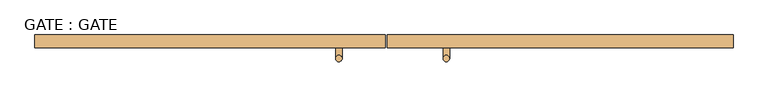
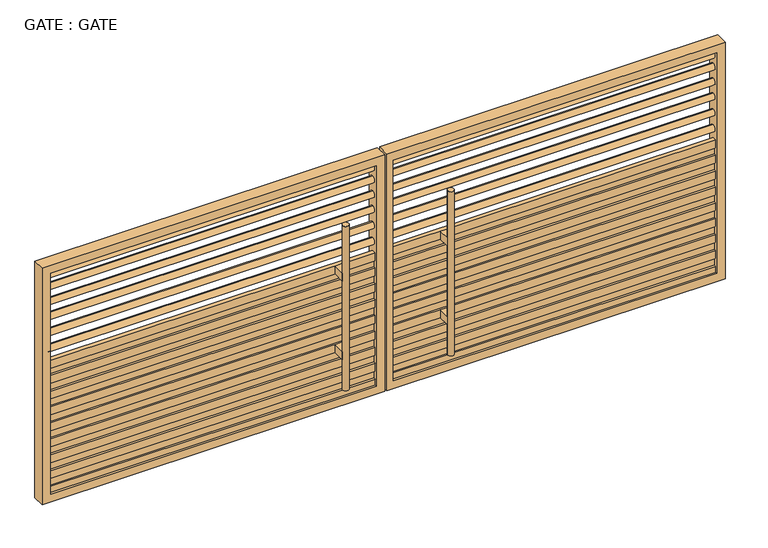
"""IFC4 building model written with IfcOpenShell, lengths in millimetres: door geometry, GATE : GATE."""

from ifc_helpers import new_model, si_unit, point, frame, frame_2d, origin, place, context, project, spatial, polyline, circle_curve, trimmed, segment, composite_curve, outline, extrude, source, transform, mapped, element, save


def gate_gate_6d9155c2(model_context):
    return source(origin(), model_context, "Body", "SweptSolid", [
        extrude(outline(composite_curve([segment(trimmed(circle_curve(frame_2d((-3297.4327882, -6020.0544725)), 19.05), [point((-3316.4827882, -6020.0544725))], [point((-3278.3827882, -6020.0544725))], False, "CARTESIAN"), True, "CONTINUOUS"), segment(trimmed(circle_curve(frame_2d((-3297.4327882, -6020.0544725)), 19.05), [point((-3278.3827882, -6020.0544725))], [point((-3316.4827882, -6020.0544725))], False, "CARTESIAN"), True, "CONTINUOUS")], self_intersect=False)), frame((0.0, 0.0, 202.6054074), z_axis=(0.0, 0.0, 1.0), x_axis=(1.0, 0.0, 0.0)), (0.0, 0.0, 1.0), 1048.3445926),
        extrude(outline(polyline([(-3278.3827882, -6020.0544725), (-3316.4827882, -6020.0544725), (-3316.4827882, -5943.8544725), (-3278.3827882, -5943.8544725), (-3278.3827882, -6020.0544725)])), frame((0.0, 0.0, 895.35), z_axis=(0.0, 0.0, 1.0), x_axis=(1.0, 0.0, 0.0)), (0.0, 0.0, 1.0), 50.8),
        extrude(outline(polyline([(-3278.3827882, -6020.0544725), (-3316.4827882, -6020.0544725), (-3316.4827882, -5943.8544725), (-3278.3827882, -5943.8544725), (-3278.3827882, -6020.0544725)])), frame((0.0, 0.0, 393.7), z_axis=(0.0, 0.0, 1.0), x_axis=(1.0, 0.0, 0.0)), (0.0, 0.0, 1.0), 50.8),
        extrude(outline(composite_curve([segment(trimmed(circle_curve(frame_2d((-3932.4327882, -6020.0544725)), 19.05), [point((-3951.4827882, -6020.0544725))], [point((-3913.3827882, -6020.0544725))], False, "CARTESIAN"), True, "CONTINUOUS"), segment(trimmed(circle_curve(frame_2d((-3932.4327882, -6020.0544725)), 19.05), [point((-3913.3827882, -6020.0544725))], [point((-3951.4827882, -6020.0544725))], False, "CARTESIAN"), True, "CONTINUOUS")], self_intersect=False)), frame((0.0, 0.0, 202.6054074), z_axis=(0.0, 0.0, 1.0), x_axis=(1.0, 0.0, 0.0)), (0.0, 0.0, 1.0), 1048.3445926),
        extrude(outline(polyline([(-3913.3827882, -6020.0544725), (-3951.4827882, -6020.0544725), (-3951.4827882, -5943.8544725), (-3913.3827882, -5943.8544725), (-3913.3827882, -6020.0544725)])), frame((0.0, 0.0, 895.35), z_axis=(0.0, 0.0, 1.0), x_axis=(1.0, 0.0, 0.0)), (0.0, 0.0, 1.0), 50.8),
        extrude(outline(polyline([(-3913.3827882, -6020.0544725), (-3951.4827882, -6020.0544725), (-3951.4827882, -5943.8544725), (-3913.3827882, -5943.8544725), (-3913.3827882, -6020.0544725)])), frame((0.0, 0.0, 393.7), z_axis=(0.0, 0.0, 1.0), x_axis=(1.0, 0.0, 0.0)), (0.0, 0.0, 1.0), 50.8),
        extrude(outline(polyline([(-5918.4544725, 946.15), (-5918.4544725, 101.6), (-5943.8544725, 101.6), (-5943.8544725, 139.7), (-5931.1544725, 139.7), (-5931.1544725, 190.5), (-5943.8544725, 190.5), (-5943.8544725, 241.3), (-5931.1544725, 241.3), (-5931.1544725, 292.1), (-5943.8544725, 292.1), (-5943.8544725, 342.9), (-5931.1544725, 342.9), (-5931.1544725, 393.7), (-5943.8544725, 393.7), (-5943.8544725, 444.5), (-5931.1544725, 444.5), (-5931.1544725, 495.3), (-5943.8544725, 495.3), (-5943.8544725, 546.1), (-5931.1544725, 546.1), (-5931.1544725, 596.9), (-5943.8544725, 596.9), (-5943.8544725, 647.7), (-5931.1544725, 647.7), (-5931.1544725, 698.5), (-5943.8544725, 698.5), (-5943.8544725, 749.3), (-5931.1544725, 749.3), (-5931.1544725, 800.1), (-5943.8544725, 800.1), (-5943.8544725, 850.9), (-5931.1544725, 850.9), (-5931.1544725, 895.35), (-5943.8544725, 895.35), (-5943.8544725, 946.15), (-5918.4544725, 946.15)])), frame((-3608.5827882, 0.0, 0.0), z_axis=(1.0, 0.0, 0.0), x_axis=(0.0, 1.0, 0.0)), (0.0, 0.0, 1.0), 1968.1845842),
        extrude(outline(composite_curve([segment(trimmed(circle_curve(frame_2d((-5918.4544725, 1479.0698991)), 20.0), [point((-5918.4544725, 1459.0698991))], [point((-5918.4544725, 1499.0698991))], False, "CARTESIAN"), True, "CONTINUOUS"), segment(trimmed(circle_curve(frame_2d((-5918.4544725, 1479.0698991)), 20.0), [point((-5918.4544725, 1499.0698991))], [point((-5918.4544725, 1459.0698991))], False, "CARTESIAN"), True, "CONTINUOUS")], self_intersect=False)), frame((-3608.5827882, 0.0, 0.0), z_axis=(1.0, 0.0, 0.0), x_axis=(0.0, 1.0, 0.0)), (0.0, 0.0, 1.0), 1968.1845842),
        extrude(outline(composite_curve([segment(trimmed(circle_curve(frame_2d((-5918.4544725, 1402.8698991)), 20.0), [point((-5918.4544725, 1382.8698991))], [point((-5918.4544725, 1422.8698991))], False, "CARTESIAN"), True, "CONTINUOUS"), segment(trimmed(circle_curve(frame_2d((-5918.4544725, 1402.8698991)), 20.0), [point((-5918.4544725, 1422.8698991))], [point((-5918.4544725, 1382.8698991))], False, "CARTESIAN"), True, "CONTINUOUS")], self_intersect=False)), frame((-3608.5827882, 0.0, 0.0), z_axis=(1.0, 0.0, 0.0), x_axis=(0.0, 1.0, 0.0)), (0.0, 0.0, 1.0), 1968.1845842),
        extrude(outline(composite_curve([segment(trimmed(circle_curve(frame_2d((-5918.4544725, 1307.6198991)), 20.0), [point((-5918.4544725, 1287.6198991))], [point((-5918.4544725, 1327.6198991))], False, "CARTESIAN"), True, "CONTINUOUS"), segment(trimmed(circle_curve(frame_2d((-5918.4544725, 1307.6198991)), 20.0), [point((-5918.4544725, 1327.6198991))], [point((-5918.4544725, 1287.6198991))], False, "CARTESIAN"), True, "CONTINUOUS")], self_intersect=False)), frame((-3608.5827882, 0.0, 0.0), z_axis=(1.0, 0.0, 0.0), x_axis=(0.0, 1.0, 0.0)), (0.0, 0.0, 1.0), 1968.1845842),
        extrude(outline(composite_curve([segment(trimmed(circle_curve(frame_2d((-5918.4544725, 1212.3698991)), 20.0), [point((-5918.4544725, 1192.3698991))], [point((-5918.4544725, 1232.3698991))], False, "CARTESIAN"), True, "CONTINUOUS"), segment(trimmed(circle_curve(frame_2d((-5918.4544725, 1212.3698991)), 20.0), [point((-5918.4544725, 1232.3698991))], [point((-5918.4544725, 1192.3698991))], False, "CARTESIAN"), True, "CONTINUOUS")], self_intersect=False)), frame((-3608.5827882, 0.0, 0.0), z_axis=(1.0, 0.0, 0.0), x_axis=(0.0, 1.0, 0.0)), (0.0, 0.0, 1.0), 1968.1845842),
        extrude(outline(composite_curve([segment(trimmed(circle_curve(frame_2d((-5918.4544725, 1110.7698991)), 20.0), [point((-5918.4544725, 1090.7698991))], [point((-5918.4544725, 1130.7698991))], False, "CARTESIAN"), True, "CONTINUOUS"), segment(trimmed(circle_curve(frame_2d((-5918.4544725, 1110.7698991)), 20.0), [point((-5918.4544725, 1130.7698991))], [point((-5918.4544725, 1090.7698991))], False, "CARTESIAN"), True, "CONTINUOUS")], self_intersect=False)), frame((-3608.5827882, 0.0, 0.0), z_axis=(1.0, 0.0, 0.0), x_axis=(0.0, 1.0, 0.0)), (0.0, 0.0, 1.0), 1968.1845842),
        extrude(outline(composite_curve([segment(trimmed(circle_curve(frame_2d((-5918.4544725, 1009.1698991)), 20.0), [point((-5918.4544725, 989.1698991))], [point((-5918.4544725, 1029.1698991))], False, "CARTESIAN"), True, "CONTINUOUS"), segment(trimmed(circle_curve(frame_2d((-5918.4544725, 1009.1698991)), 20.0), [point((-5918.4544725, 1029.1698991))], [point((-5918.4544725, 989.1698991))], False, "CARTESIAN"), True, "CONTINUOUS")], self_intersect=False)), frame((-3608.5827882, 0.0, 0.0), z_axis=(1.0, 0.0, 0.0), x_axis=(0.0, 1.0, 0.0)), (0.0, 0.0, 1.0), 1968.1845842),
        extrude(outline(polyline([(-5918.4544725, 946.15), (-5918.4544725, 101.6), (-5943.8544725, 101.6), (-5943.8544725, 139.7), (-5931.1544725, 139.7), (-5931.1544725, 190.5), (-5943.8544725, 190.5), (-5943.8544725, 241.3), (-5931.1544725, 241.3), (-5931.1544725, 292.1), (-5943.8544725, 292.1), (-5943.8544725, 342.9), (-5931.1544725, 342.9), (-5931.1544725, 393.7), (-5943.8544725, 393.7), (-5943.8544725, 444.5), (-5931.1544725, 444.5), (-5931.1544725, 495.3), (-5943.8544725, 495.3), (-5943.8544725, 546.1), (-5931.1544725, 546.1), (-5931.1544725, 596.9), (-5943.8544725, 596.9), (-5943.8544725, 647.7), (-5931.1544725, 647.7), (-5931.1544725, 698.5), (-5943.8544725, 698.5), (-5943.8544725, 749.3), (-5931.1544725, 749.3), (-5931.1544725, 800.1), (-5943.8544725, 800.1), (-5943.8544725, 850.9), (-5931.1544725, 850.9), (-5931.1544725, 895.35), (-5943.8544725, 895.35), (-5943.8544725, 946.15), (-5918.4544725, 946.15)])), frame((-5678.3673724, 0.0, 0.0), z_axis=(1.0, 0.0, 0.0), x_axis=(0.0, 1.0, 0.0)), (0.0, 0.0, 1.0), 1968.1845842),
        extrude(outline(composite_curve([segment(trimmed(circle_curve(frame_2d((-5918.4544725, 1479.0698991)), 20.0), [point((-5918.4544725, 1459.0698991))], [point((-5918.4544725, 1499.0698991))], False, "CARTESIAN"), True, "CONTINUOUS"), segment(trimmed(circle_curve(frame_2d((-5918.4544725, 1479.0698991)), 20.0), [point((-5918.4544725, 1499.0698991))], [point((-5918.4544725, 1459.0698991))], False, "CARTESIAN"), True, "CONTINUOUS")], self_intersect=False)), frame((-5678.3673724, 0.0, 0.0), z_axis=(1.0, 0.0, 0.0), x_axis=(0.0, 1.0, 0.0)), (0.0, 0.0, 1.0), 1968.1845842),
        extrude(outline(composite_curve([segment(trimmed(circle_curve(frame_2d((-5918.4544725, 1402.8698991)), 20.0), [point((-5918.4544725, 1382.8698991))], [point((-5918.4544725, 1422.8698991))], False, "CARTESIAN"), True, "CONTINUOUS"), segment(trimmed(circle_curve(frame_2d((-5918.4544725, 1402.8698991)), 20.0), [point((-5918.4544725, 1422.8698991))], [point((-5918.4544725, 1382.8698991))], False, "CARTESIAN"), True, "CONTINUOUS")], self_intersect=False)), frame((-5678.3673724, 0.0, 0.0), z_axis=(1.0, 0.0, 0.0), x_axis=(0.0, 1.0, 0.0)), (0.0, 0.0, 1.0), 1968.1845842),
        extrude(outline(composite_curve([segment(trimmed(circle_curve(frame_2d((-5918.4544725, 1307.6198991)), 20.0), [point((-5918.4544725, 1287.6198991))], [point((-5918.4544725, 1327.6198991))], False, "CARTESIAN"), True, "CONTINUOUS"), segment(trimmed(circle_curve(frame_2d((-5918.4544725, 1307.6198991)), 20.0), [point((-5918.4544725, 1327.6198991))], [point((-5918.4544725, 1287.6198991))], False, "CARTESIAN"), True, "CONTINUOUS")], self_intersect=False)), frame((-5678.3673724, 0.0, 0.0), z_axis=(1.0, 0.0, 0.0), x_axis=(0.0, 1.0, 0.0)), (0.0, 0.0, 1.0), 1968.1845842),
        extrude(outline(composite_curve([segment(trimmed(circle_curve(frame_2d((-5918.4544725, 1212.3698991)), 20.0), [point((-5918.4544725, 1192.3698991))], [point((-5918.4544725, 1232.3698991))], False, "CARTESIAN"), True, "CONTINUOUS"), segment(trimmed(circle_curve(frame_2d((-5918.4544725, 1212.3698991)), 20.0), [point((-5918.4544725, 1232.3698991))], [point((-5918.4544725, 1192.3698991))], False, "CARTESIAN"), True, "CONTINUOUS")], self_intersect=False)), frame((-5678.3673724, 0.0, 0.0), z_axis=(1.0, 0.0, 0.0), x_axis=(0.0, 1.0, 0.0)), (0.0, 0.0, 1.0), 1968.1845842),
        extrude(outline(composite_curve([segment(trimmed(circle_curve(frame_2d((-5918.4544725, 1110.7698991)), 20.0), [point((-5918.4544725, 1090.7698991))], [point((-5918.4544725, 1130.7698991))], False, "CARTESIAN"), True, "CONTINUOUS"), segment(trimmed(circle_curve(frame_2d((-5918.4544725, 1110.7698991)), 20.0), [point((-5918.4544725, 1130.7698991))], [point((-5918.4544725, 1090.7698991))], False, "CARTESIAN"), True, "CONTINUOUS")], self_intersect=False)), frame((-5678.3673724, 0.0, 0.0), z_axis=(1.0, 0.0, 0.0), x_axis=(0.0, 1.0, 0.0)), (0.0, 0.0, 1.0), 1968.1845842),
        extrude(outline(composite_curve([segment(trimmed(circle_curve(frame_2d((-5918.4544725, 1009.1698991)), 20.0), [point((-5918.4544725, 989.1698991))], [point((-5918.4544725, 1029.1698991))], False, "CARTESIAN"), True, "CONTINUOUS"), segment(trimmed(circle_curve(frame_2d((-5918.4544725, 1009.1698991)), 20.0), [point((-5918.4544725, 1029.1698991))], [point((-5918.4544725, 989.1698991))], False, "CARTESIAN"), True, "CONTINUOUS")], self_intersect=False)), frame((-5678.3673724, 0.0, 0.0), z_axis=(1.0, 0.0, 0.0), x_axis=(0.0, 1.0, 0.0)), (0.0, 0.0, 1.0), 1968.1845842),
        extrude(outline(polyline([(1561.6198991, -3646.6827882), (50.8, -3646.6827882), (50.8, -1602.2982041), (1561.6198991, -1602.2982041), (1561.6198991, -3646.6827882)]), holes=[polyline([(101.6, -1653.0982041), (101.6, -3608.5827882), (1510.8198991, -3608.5827882), (1510.8198991, -1653.0982041), (101.6, -1653.0982041)])]), frame((0.0, -5956.5544725, 0.0), z_axis=(0.0, 1.0, 0.0), x_axis=(0.0, 0.0, 1.0)), (0.0, 0.0, 1.0), 76.2),
        extrude(outline(polyline([(50.8, -3659.3827882), (1561.6198991, -3659.3827882), (1561.6198991, -5729.1673724), (50.8, -5729.1673724), (50.8, -3659.3827882)]), holes=[polyline([(1510.8198991, -3710.1827882), (101.6, -3710.1827882), (101.6, -5678.3673724), (1510.8198991, -5678.3673724), (1510.8198991, -3710.1827882)])]), frame((0.0, -5956.5544725, 0.0), z_axis=(0.0, 1.0, 0.0), x_axis=(0.0, 0.0, 1.0)), (0.0, 0.0, 1.0), 76.2),
    ])


if __name__ == "__main__":
    model = new_model("IFC4")
    model_context = context("Model", 3, world=origin())
    ifc_project = project(units=[si_unit("LENGTHUNIT", "METRE", prefix="MILLI")], contexts=[model_context])
    site = spatial("IfcSite", under=ifc_project)
    building = spatial("IfcBuilding", under=site)
    placement = place(None, origin())
    gate_gate_shape = gate_gate_6d9155c2(model_context)
    element("IfcDoor", 1, ObjectType="GATE : GATE", at=placement, inside=building, context=model_context, shape_type="MappedRepresentation", body=[
        mapped(gate_gate_shape, transform((0.0, 0.0, 0.0), x_axis=(1.0, 0.0, 0.0), y_axis=(0.0, 1.0, 0.0), z_axis=(0.0, 0.0, 1.0))),
    ])
    save(model, "model.ifc")

# Revit data of these elements
# Type "GATE : GATE"
#   Type Mark = "11"
# Element 1 (IfcDoor, "GATE : GATE")
#   Materials on its faces: "Door - Panel", "Iron, Ductile", "Aluminum"
# Materials
#   "Door - Panel": class "Wood", colour RGB 210 159 95, transparency 0, Cost = 0
#   "Iron, Ductile": class "Metal", colour RGB 0 0 0, transparency 0, Description = "Ductile cast iron", Cost = 0
#   "Aluminum": class "Metal", colour RGB 247 247 247, transparency 0, Description = "Aluminum 6061", Cost = 0
